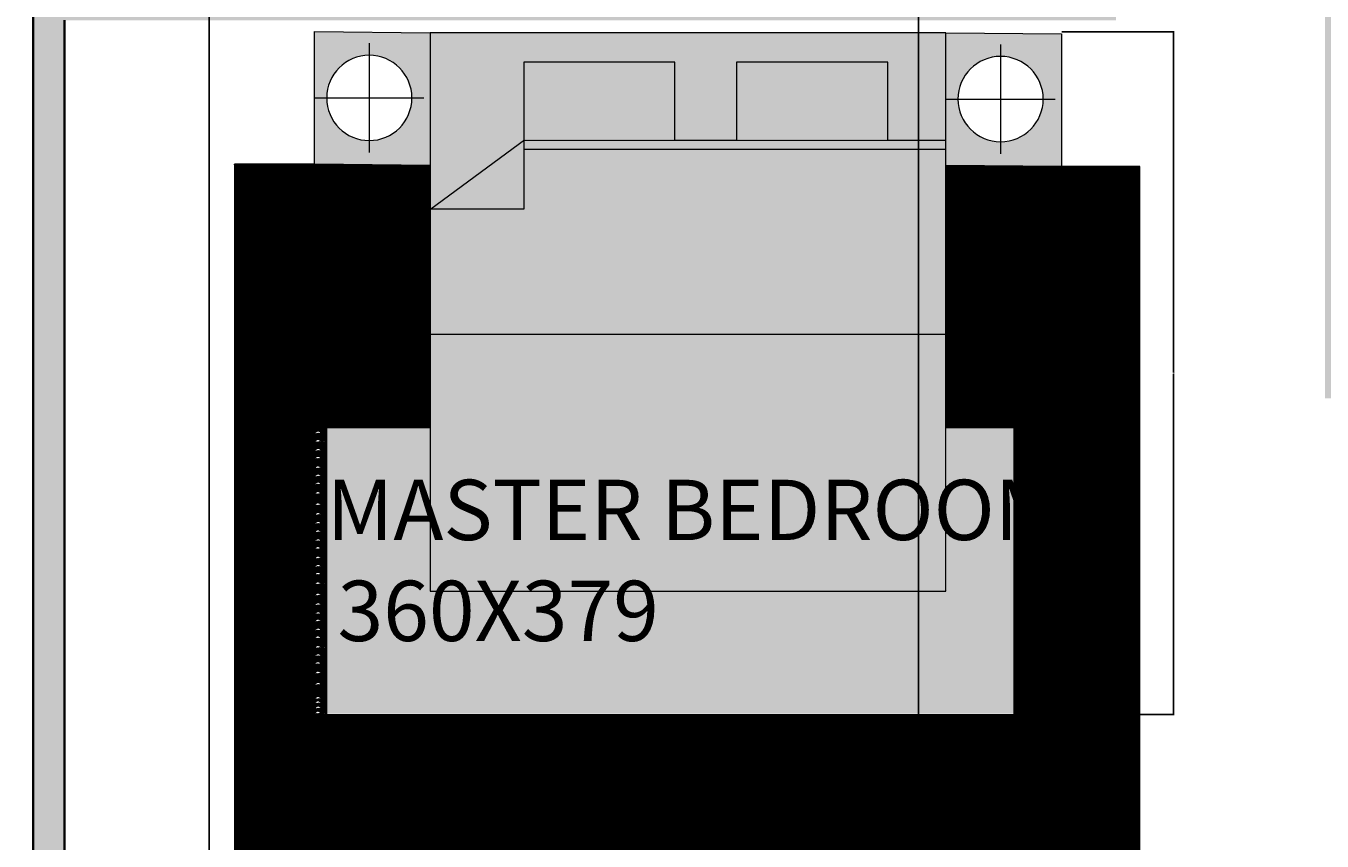
# Model space of a CAD drawing. Units: inches. Extents: x 192 to 1361, y -1362 to 367.
# Tile 21 of 23: x 783 to 1153, y -304 to -71. Entities that reach past the tile are written whole.
import ezdxf

# ---------------------------------------------------------------- set-up
doc = ezdxf.new("R2010")
doc.units = ezdxf.units.IN
doc.header["$MEASUREMENT"] = 0
for name, color, linetype, lineweight in [('A-ANNO-DIMS', 2, 'Continuous', 18), ('A-AREA-IDEN', 7, 'Continuous', 18), ('A-FLOR', 8, 'Continuous', 18), ('A-WALL-PATT', 250, 'Continuous', 13), ('furniture', 32, 'Continuous', 18), ('walls', 7, 'Continuous', 35)]:
    doc.layers.add(name, color=color, linetype=linetype, lineweight=lineweight)
doc.layers.add('A-FLOR-PATT', color=254, linetype='Continuous', lineweight=13, true_color=0xfeeab9)
doc.layers.add('A-FURN-PATT', color=254, linetype='Continuous', lineweight=13, true_color=0xfeeab9)
doc.styles.get("Standard").update_dxf_attribs({"font": 'arial.ttf'})
doc.dimstyles.get("Standard").update_dxf_attribs({"dimtxt": 0.18, "dimasz": 0.18, "dimexe": 0.18, "dimexo": 0.0625, "dimgap": 0.09, "dimtad": 0, "dimtih": 1, "dimtoh": 1, "dimzin": 0, "dimdsep": 46, "dimlunit": 3, "dimtxsty": 'Standard', "dimcen": 0.09, "dimadec": 0, "dimazin": 0, "dimtfac": 1, "dimtofl": 0, "dimtmove": 0, "dimatfit": 3, "dimfxl": 1, "dimtolj": 1, "dimtzin": 0, "dimarcsym": 0})

# ---------------------------------------------------------------- blocks, each defined once
blk = doc.blocks.new('CARPET')
at = {"layer": 'furniture'}
for p, q in [((-51.53, -98.11), (-51.53, -55.12)), ((-51.53, -55.12), (-41.27, -55.12)), ((36, -55.12), (51.55, -55.12)), ((51.55, -55.12), (51.55, -98.11)), ((51.55, -98.11), (-51.53, -98.11))]:
    blk.add_line(p, q, dxfattribs=at)
for points, knots in [([(-53.37, -55.99), (-53.22, -55.8), (-52.9, -55.41), (-52.34, -55.8), (-51.89, -56.08), (-51.65, -55.91), (-51.53, -55.83)], [0, 0, 0, 0, 0.653278, 1.290138, 1.740457, 2.114451, 2.114451, 2.114451, 2.114451]), ([(53.37, -55.99), (53.22, -55.8), (52.9, -55.41), (52.34, -55.8), (51.89, -56.08), (51.65, -55.91), (51.53, -55.83)], [0, 0, 0, 0, 0.653278, 1.290138, 1.740457, 2.114451, 2.114451, 2.114451, 2.114451]), ([(-53.37, -57.26), (-53.22, -57.07), (-52.9, -56.67), (-52.34, -57.07), (-51.89, -57.35), (-51.65, -57.17), (-51.53, -57.1)], [0, 0, 0, 0, 0.653278, 1.290138, 1.740457, 2.114451, 2.114451, 2.114451, 2.114451]), ([(-53.37, -58.59), (-53.22, -58.4), (-52.9, -58.01), (-52.34, -58.4), (-51.89, -58.68), (-51.65, -58.5), (-51.53, -58.43)], [0, 0, 0, 0, 0.653278, 1.290138, 1.740457, 2.114451, 2.114451, 2.114451, 2.114451]), ([(53.37, -57.26), (53.22, -57.07), (52.9, -56.67), (52.34, -57.07), (51.89, -57.35), (51.65, -57.17), (51.53, -57.1)], [0, 0, 0, 0, 0.653278, 1.290138, 1.740457, 2.114451, 2.114451, 2.114451, 2.114451]), ([(53.37, -58.59), (53.22, -58.4), (52.9, -58.01), (52.34, -58.4), (51.89, -58.68), (51.65, -58.5), (51.53, -58.43)], [0, 0, 0, 0, 0.653278, 1.290138, 1.740457, 2.114451, 2.114451, 2.114451, 2.114451]), ([(-53.37, -59.78), (-53.22, -59.58), (-52.9, -59.19), (-52.34, -59.58), (-51.89, -59.86), (-51.65, -59.69), (-51.53, -59.61)], [0, 0, 0, 0, 0.653278, 1.290138, 1.740457, 2.114451, 2.114451, 2.114451, 2.114451]), ([(53.37, -59.78), (53.22, -59.58), (52.9, -59.19), (52.34, -59.58), (51.89, -59.86), (51.65, -59.69), (51.53, -59.61)], [0, 0, 0, 0, 0.653278, 1.290138, 1.740457, 2.114451, 2.114451, 2.114451, 2.114451]), ([(-53.37, -61.22), (-53.22, -61.02), (-52.9, -60.63), (-52.34, -61.02), (-51.89, -61.3), (-51.65, -61.13), (-51.53, -61.05)], [0, 0, 0, 0, 0.653278, 1.290138, 1.740457, 2.114451, 2.114451, 2.114451, 2.114451]), ([(-53.37, -62.44), (-53.22, -62.25), (-52.9, -61.86), (-52.34, -62.25), (-51.89, -62.53), (-51.65, -62.36), (-51.53, -62.28)], [0, 0, 0, 0, 0.653278, 1.290138, 1.740457, 2.114451, 2.114451, 2.114451, 2.114451]), ([(53.37, -61.22), (53.22, -61.02), (52.9, -60.63), (52.34, -61.02), (51.89, -61.3), (51.65, -61.13), (51.53, -61.05)], [0, 0, 0, 0, 0.653278, 1.290138, 1.740457, 2.114451, 2.114451, 2.114451, 2.114451]), ([(53.37, -62.44), (53.22, -62.25), (52.9, -61.86), (52.34, -62.25), (51.89, -62.53), (51.65, -62.36), (51.53, -62.28)], [0, 0, 0, 0, 0.653278, 1.290138, 1.740457, 2.114451, 2.114451, 2.114451, 2.114451]), ([(-53.37, -63.63), (-53.22, -63.43), (-52.9, -63.04), (-52.34, -63.43), (-51.89, -63.72), (-51.65, -63.54), (-51.53, -63.46)], [0, 0, 0, 0, 0.653278, 1.290138, 1.740457, 2.114451, 2.114451, 2.114451, 2.114451]), ([(53.37, -63.63), (53.22, -63.43), (52.9, -63.04), (52.34, -63.43), (51.89, -63.72), (51.65, -63.54), (51.53, -63.46)], [0, 0, 0, 0, 0.653278, 1.290138, 1.740457, 2.114451, 2.114451, 2.114451, 2.114451]), ([(-53.37, -65.07), (-53.22, -64.87), (-52.9, -64.48), (-52.34, -64.87), (-51.89, -65.15), (-51.65, -64.98), (-51.53, -64.9)], [0, 0, 0, 0, 0.653278, 1.290138, 1.740457, 2.114451, 2.114451, 2.114451, 2.114451]), ([(53.37, -65.07), (53.22, -64.87), (52.9, -64.48), (52.34, -64.87), (51.89, -65.15), (51.65, -64.98), (51.53, -64.9)], [0, 0, 0, 0, 0.653278, 1.290138, 1.740457, 2.114451, 2.114451, 2.114451, 2.114451]), ([(-53.37, -66.76), (-53.22, -66.56), (-52.9, -66.17), (-52.34, -66.56), (-51.89, -66.84), (-51.65, -66.67), (-51.53, -66.59)], [0, 0, 0, 0, 0.653278, 1.290138, 1.740457, 2.114451, 2.114451, 2.114451, 2.114451]), ([(-53.37, -68.2), (-53.22, -68), (-52.9, -67.61), (-52.34, -68), (-51.89, -68.28), (-51.65, -68.11), (-51.53, -68.03)], [0, 0, 0, 0, 0.653278, 1.290138, 1.740457, 2.114451, 2.114451, 2.114451, 2.114451]), ([(53.37, -66.76), (53.22, -66.56), (52.9, -66.17), (52.34, -66.56), (51.89, -66.84), (51.65, -66.67), (51.53, -66.59)], [0, 0, 0, 0, 0.653278, 1.290138, 1.740457, 2.114451, 2.114451, 2.114451, 2.114451]), ([(53.37, -68.2), (53.22, -68), (52.9, -67.61), (52.34, -68), (51.89, -68.28), (51.65, -68.11), (51.53, -68.03)], [0, 0, 0, 0, 0.653278, 1.290138, 1.740457, 2.114451, 2.114451, 2.114451, 2.114451]), ([(-53.37, -69.53), (-53.22, -69.33), (-52.9, -68.94), (-52.34, -69.33), (-51.89, -69.61), (-51.65, -69.44), (-51.53, -69.36)], [0, 0, 0, 0, 0.653278, 1.290138, 1.740457, 2.114451, 2.114451, 2.114451, 2.114451]), ([(53.37, -69.53), (53.22, -69.33), (52.9, -68.94), (52.34, -69.33), (51.89, -69.61), (51.65, -69.44), (51.53, -69.36)], [0, 0, 0, 0, 0.653278, 1.290138, 1.740457, 2.114451, 2.114451, 2.114451, 2.114451]), ([(-53.37, -70.79), (-53.22, -70.6), (-52.9, -70.21), (-52.34, -70.6), (-51.89, -70.88), (-51.65, -70.7), (-51.53, -70.63)], [0, 0, 0, 0, 0.653278, 1.290138, 1.740457, 2.114451, 2.114451, 2.114451, 2.114451]), ([(-53.37, -72.12), (-53.22, -71.93), (-52.9, -71.54), (-52.34, -71.93), (-51.89, -72.21), (-51.65, -72.04), (-51.53, -71.96)], [0, 0, 0, 0, 0.653278, 1.290138, 1.740457, 2.114451, 2.114451, 2.114451, 2.114451]), ([(53.37, -70.79), (53.22, -70.6), (52.9, -70.21), (52.34, -70.6), (51.89, -70.88), (51.65, -70.7), (51.53, -70.63)], [0, 0, 0, 0, 0.653278, 1.290138, 1.740457, 2.114451, 2.114451, 2.114451, 2.114451]), ([(53.37, -72.12), (53.22, -71.93), (52.9, -71.54), (52.34, -71.93), (51.89, -72.21), (51.65, -72.04), (51.53, -71.96)], [0, 0, 0, 0, 0.653278, 1.290138, 1.740457, 2.114451, 2.114451, 2.114451, 2.114451]), ([(-53.37, -73.31), (-53.22, -73.11), (-52.9, -72.72), (-52.34, -73.11), (-51.89, -73.4), (-51.65, -73.22), (-51.53, -73.14)], [0, 0, 0, 0, 0.653278, 1.290138, 1.740457, 2.114451, 2.114451, 2.114451, 2.114451]), ([(53.37, -73.31), (53.22, -73.11), (52.9, -72.72), (52.34, -73.11), (51.89, -73.4), (51.65, -73.22), (51.53, -73.14)], [0, 0, 0, 0, 0.653278, 1.290138, 1.740457, 2.114451, 2.114451, 2.114451, 2.114451]), ([(-53.37, -74.75), (-53.22, -74.55), (-52.9, -74.16), (-52.34, -74.55), (-51.89, -74.83), (-51.65, -74.66), (-51.53, -74.58)], [0, 0, 0, 0, 0.653278, 1.290138, 1.740457, 2.114451, 2.114451, 2.114451, 2.114451]), ([(-53.37, -75.98), (-53.22, -75.78), (-52.9, -75.39), (-52.34, -75.78), (-51.89, -76.06), (-51.65, -75.89), (-51.53, -75.81)], [0, 0, 0, 0, 0.653278, 1.290138, 1.740457, 2.114451, 2.114451, 2.114451, 2.114451]), ([(53.37, -74.75), (53.22, -74.55), (52.9, -74.16), (52.34, -74.55), (51.89, -74.83), (51.65, -74.66), (51.53, -74.58)], [0, 0, 0, 0, 0.653278, 1.290138, 1.740457, 2.114451, 2.114451, 2.114451, 2.114451]), ([(53.37, -75.98), (53.22, -75.78), (52.9, -75.39), (52.34, -75.78), (51.89, -76.06), (51.65, -75.89), (51.53, -75.81)], [0, 0, 0, 0, 0.653278, 1.290138, 1.740457, 2.114451, 2.114451, 2.114451, 2.114451]), ([(-53.37, -77.16), (-53.22, -76.96), (-52.9, -76.57), (-52.34, -76.96), (-51.89, -77.25), (-51.65, -77.07), (-51.53, -76.99)], [0, 0, 0, 0, 0.653278, 1.290138, 1.740457, 2.114451, 2.114451, 2.114451, 2.114451]), ([(53.37, -77.16), (53.22, -76.96), (52.9, -76.57), (52.34, -76.96), (51.89, -77.25), (51.65, -77.07), (51.53, -76.99)], [0, 0, 0, 0, 0.653278, 1.290138, 1.740457, 2.114451, 2.114451, 2.114451, 2.114451]), ([(-53.37, -78.6), (-53.22, -78.4), (-52.9, -78.01), (-52.34, -78.4), (-51.89, -78.68), (-51.65, -78.51), (-51.53, -78.43)], [0, 0, 0, 0, 0.653278, 1.290138, 1.740457, 2.114451, 2.114451, 2.114451, 2.114451]), ([(53.37, -78.6), (53.22, -78.4), (52.9, -78.01), (52.34, -78.4), (51.89, -78.68), (51.65, -78.51), (51.53, -78.43)], [0, 0, 0, 0, 0.653278, 1.290138, 1.740457, 2.114451, 2.114451, 2.114451, 2.114451]), ([(-53.37, -80.29), (-53.22, -80.09), (-52.9, -79.7), (-52.34, -80.09), (-51.89, -80.37), (-51.65, -80.2), (-51.53, -80.12)], [0, 0, 0, 0, 0.653278, 1.290138, 1.740457, 2.114451, 2.114451, 2.114451, 2.114451]), ([(-53.37, -81.73), (-53.22, -81.53), (-52.9, -81.14), (-52.34, -81.53), (-51.89, -81.81), (-51.65, -81.64), (-51.53, -81.56)], [0, 0, 0, 0, 0.653278, 1.290138, 1.740457, 2.114451, 2.114451, 2.114451, 2.114451]), ([(53.37, -80.29), (53.22, -80.09), (52.9, -79.7), (52.34, -80.09), (51.89, -80.37), (51.65, -80.2), (51.53, -80.12)], [0, 0, 0, 0, 0.653278, 1.290138, 1.740457, 2.114451, 2.114451, 2.114451, 2.114451]), ([(53.37, -81.73), (53.22, -81.53), (52.9, -81.14), (52.34, -81.53), (51.89, -81.81), (51.65, -81.64), (51.53, -81.56)], [0, 0, 0, 0, 0.653278, 1.290138, 1.740457, 2.114451, 2.114451, 2.114451, 2.114451]), ([(-53.37, -83.06), (-53.22, -82.86), (-52.9, -82.47), (-52.34, -82.86), (-51.89, -83.14), (-51.65, -82.97), (-51.53, -82.89)], [0, 0, 0, 0, 0.653278, 1.290138, 1.740457, 2.114451, 2.114451, 2.114451, 2.114451]), ([(53.37, -83.06), (53.22, -82.86), (52.9, -82.47), (52.34, -82.86), (51.89, -83.14), (51.65, -82.97), (51.53, -82.89)], [0, 0, 0, 0, 0.653278, 1.290138, 1.740457, 2.114451, 2.114451, 2.114451, 2.114451]), ([(-53.37, -84.18), (-53.22, -83.99), (-52.9, -83.6), (-52.34, -83.99), (-51.89, -84.27), (-51.65, -84.09), (-51.53, -84.02)], [0, 0, 0, 0, 0.653278, 1.290138, 1.740457, 2.114451, 2.114451, 2.114451, 2.114451]), ([(-53.37, -85.51), (-53.22, -85.32), (-52.9, -84.93), (-52.34, -85.32), (-51.89, -85.6), (-51.65, -85.42), (-51.53, -85.35)], [0, 0, 0, 0, 0.653278, 1.290138, 1.740457, 2.114451, 2.114451, 2.114451, 2.114451]), ([(53.37, -84.18), (53.22, -83.99), (52.9, -83.6), (52.34, -83.99), (51.89, -84.27), (51.65, -84.09), (51.53, -84.02)], [0, 0, 0, 0, 0.653278, 1.290138, 1.740457, 2.114451, 2.114451, 2.114451, 2.114451]), ([(53.37, -85.51), (53.22, -85.32), (52.9, -84.93), (52.34, -85.32), (51.89, -85.6), (51.65, -85.42), (51.53, -85.35)], [0, 0, 0, 0, 0.653278, 1.290138, 1.740457, 2.114451, 2.114451, 2.114451, 2.114451]), ([(-53.37, -86.7), (-53.22, -86.5), (-52.9, -86.11), (-52.34, -86.5), (-51.89, -86.78), (-51.65, -86.61), (-51.53, -86.53)], [0, 0, 0, 0, 0.653278, 1.290138, 1.740457, 2.114451, 2.114451, 2.114451, 2.114451]), ([(53.37, -86.7), (53.22, -86.5), (52.9, -86.11), (52.34, -86.5), (51.89, -86.78), (51.65, -86.61), (51.53, -86.53)], [0, 0, 0, 0, 0.653278, 1.290138, 1.740457, 2.114451, 2.114451, 2.114451, 2.114451]), ([(-53.37, -88.14), (-53.22, -87.94), (-52.9, -87.55), (-52.34, -87.94), (-51.89, -88.22), (-51.65, -88.05), (-51.53, -87.97)], [0, 0, 0, 0, 0.653278, 1.290138, 1.740457, 2.114451, 2.114451, 2.114451, 2.114451]), ([(-53.37, -89.36), (-53.22, -89.17), (-52.9, -88.78), (-52.34, -89.17), (-51.89, -89.45), (-51.65, -89.28), (-51.53, -89.2)], [0, 0, 0, 0, 0.653278, 1.290138, 1.740457, 2.114451, 2.114451, 2.114451, 2.114451]), ([(53.37, -88.14), (53.22, -87.94), (52.9, -87.55), (52.34, -87.94), (51.89, -88.22), (51.65, -88.05), (51.53, -87.97)], [0, 0, 0, 0, 0.653278, 1.290138, 1.740457, 2.114451, 2.114451, 2.114451, 2.114451]), ([(53.37, -89.36), (53.22, -89.17), (52.9, -88.78), (52.34, -89.17), (51.89, -89.45), (51.65, -89.28), (51.53, -89.2)], [0, 0, 0, 0, 0.653278, 1.290138, 1.740457, 2.114451, 2.114451, 2.114451, 2.114451]), ([(-53.37, -90.55), (-53.22, -90.35), (-52.9, -89.96), (-52.34, -90.35), (-51.89, -90.64), (-51.65, -90.46), (-51.53, -90.38)], [0, 0, 0, 0, 0.653278, 1.290138, 1.740457, 2.114451, 2.114451, 2.114451, 2.114451]), ([(53.37, -90.55), (53.22, -90.35), (52.9, -89.96), (52.34, -90.35), (51.9, -90.63), (51.66, -90.47), (51.55, -90.4)], [0, 0, 0, 0, 0.653278, 1.290138, 1.740457, 2.0926, 2.0926, 2.0926, 2.0926]), ([(-53.37, -91.99), (-53.22, -91.79), (-52.9, -91.4), (-52.34, -91.79), (-51.89, -92.07), (-51.65, -91.9), (-51.53, -91.82)], [0, 0, 0, 0, 0.653278, 1.290138, 1.740457, 2.114451, 2.114451, 2.114451, 2.114451]), ([(-53.37, -92.69), (-53.22, -92.48), (-52.9, -92.08), (-52.35, -92.49), (-51.89, -92.77), (-51.65, -92.6), (-51.53, -92.52)], [0, 0, 0, 0, 0.663904, 1.307406, 1.757725, 2.131719, 2.131719, 2.131719, 2.131719]), ([(-53.37, -93.61), (-53.22, -93.42), (-52.9, -93.03), (-52.34, -93.42), (-51.89, -93.7), (-51.65, -93.52), (-51.53, -93.45)], [0, 0, 0, 0, 0.653278, 1.290138, 1.740457, 2.114451, 2.114451, 2.114451, 2.114451]), ([(53.37, -91.99), (53.22, -91.79), (52.9, -91.4), (52.34, -91.79), (51.9, -92.07), (51.66, -91.91), (51.55, -91.83)], [0, 0, 0, 0, 0.653278, 1.290138, 1.740457, 2.0926, 2.0926, 2.0926, 2.0926]), ([(53.37, -92.69), (53.22, -92.49), (52.9, -92.09), (52.34, -92.49), (51.9, -92.77), (51.66, -92.61), (51.55, -92.53)], [0, 0, 0, 0, 0.656792, 1.295826, 1.746145, 2.098292, 2.098292, 2.098292, 2.098292]), ([(53.37, -93.66), (53.22, -93.46), (52.9, -93.07), (52.34, -93.46), (51.9, -93.74), (51.66, -93.58), (51.55, -93.5)], [0, 0, 0, 0, 0.653278, 1.290138, 1.740457, 2.0926, 2.0926, 2.0926, 2.0926]), ([(-53.37, -94.55), (-53.22, -94.35), (-52.9, -93.96), (-52.34, -94.35), (-51.89, -94.63), (-51.65, -94.46), (-51.53, -94.38)], [0, 0, 0, 0, 0.653278, 1.290138, 1.740457, 2.114451, 2.114451, 2.114451, 2.114451]), ([(-53.37, -95.05), (-53.22, -94.85), (-52.9, -94.46), (-52.34, -94.85), (-51.89, -95.14), (-51.65, -94.96), (-51.53, -94.88)], [0, 0, 0, 0, 0.653278, 1.290138, 1.740457, 2.114451, 2.114451, 2.114451, 2.114451]), ([(53.37, -94.59), (53.22, -94.4), (52.9, -94.01), (52.34, -94.4), (51.9, -94.68), (51.66, -94.51), (51.55, -94.44)], [0, 0, 0, 0, 0.653278, 1.290138, 1.740457, 2.0926, 2.0926, 2.0926, 2.0926]), ([(53.37, -95.1), (53.22, -94.9), (52.9, -94.51), (52.34, -94.9), (51.9, -95.18), (51.66, -95.02), (51.55, -94.94)], [0, 0, 0, 0, 0.653278, 1.290138, 1.740457, 2.0926, 2.0926, 2.0926, 2.0926]), ([(-53.37, -95.73), (-53.22, -95.54), (-52.9, -95.15), (-52.34, -95.54), (-51.89, -95.82), (-51.65, -95.65), (-51.53, -95.57)], [0, 0, 0, 0, 0.653278, 1.290138, 1.740457, 2.114451, 2.114451, 2.114451, 2.114451]), ([(-53.37, -96.38), (-53.22, -96.18), (-52.9, -95.79), (-52.34, -96.18), (-51.89, -96.47), (-51.65, -96.29), (-51.53, -96.21)], [0, 0, 0, 0, 0.653278, 1.290138, 1.740457, 2.114451, 2.114451, 2.114451, 2.114451]), ([(-53.37, -97.17), (-53.22, -96.98), (-52.9, -96.59), (-52.34, -96.98), (-51.89, -97.26), (-51.65, -97.08), (-51.53, -97.01)], [0, 0, 0, 0, 0.653278, 1.290138, 1.740457, 2.114451, 2.114451, 2.114451, 2.114451]), ([(53.37, -95.78), (53.22, -95.58), (52.9, -95.19), (52.34, -95.58), (51.89, -95.86), (51.65, -95.69), (51.53, -95.61)], [0, 0, 0, 0, 0.653278, 1.290138, 1.740457, 2.114451, 2.114451, 2.114451, 2.114451]), ([(53.37, -96.43), (53.22, -96.23), (52.9, -95.84), (52.34, -96.23), (51.89, -96.51), (51.65, -96.34), (51.53, -96.26)], [0, 0, 0, 0, 0.653278, 1.290138, 1.740457, 2.114451, 2.114451, 2.114451, 2.114451]), ([(53.37, -97.22), (53.22, -97.02), (52.9, -96.63), (52.34, -97.02), (51.89, -97.3), (51.65, -97.13), (51.53, -97.05)], [0, 0, 0, 0, 0.653278, 1.290138, 1.740457, 2.114451, 2.114451, 2.114451, 2.114451]), ([(-53.37, -97.99), (-53.22, -97.79), (-52.9, -97.4), (-52.34, -97.79), (-51.89, -98.08), (-51.65, -97.9), (-51.53, -97.82)], [0, 0, 0, 0, 0.653278, 1.290138, 1.740457, 2.114451, 2.114451, 2.114451, 2.114451]), ([(53.37, -97.99), (53.22, -97.79), (52.9, -97.4), (52.34, -97.79), (51.89, -98.08), (51.65, -97.9), (51.53, -97.82)], [0, 0, 0, 0, 0.653278, 1.290138, 1.740457, 2.114451, 2.114451, 2.114451, 2.114451])]:
    blk.add_open_spline(points, degree=3, knots=knots, dxfattribs=at)
blk = doc.blocks.new('A$C58D270C6')
at = {"layer": 'furniture'}
for p, q in [((9.09, 124.13), (9.09, 108.87)), ((1.46, 116.5), (16.73, 116.5)), ((14.97, 94.84), (24.62, 107.92)), ((24.62, 94.93), (24.62, 107.92)), ((42.08, 108), (42.08, 36)), ((14.97, 94.93), (24.62, 94.93)), ((14.97, 94.84), (14.97, 36)), ((16.22, 94.93), (16.22, 36)), ((9.25, 36), (9.25, 20.74)), ((1.62, 28.37), (16.88, 28.37))]:
    blk.add_line(p, q, dxfattribs=at)
for points in [[(18.5, 108), (18.34, 124.13), (-0.16, 124.13), (0, 108)], [(0, 108), (77.91, 108), (77.91, 36), (0, 36)], [(4.09, 94.93), (14.97, 94.93), (14.97, 73.83), (4.09, 73.83)], [(4.09, 65.23), (14.97, 65.23), (14.97, 44.13), (4.09, 44.13)], [(18.65, 19.87), (18.5, 36), (0, 36), (0.16, 19.87)]]:
    blk.add_lwpolyline(points, close=True, dxfattribs=at)
for centre in [(9.09, 116.5), (9.25, 28.37)]:
    blk.add_circle(centre, 5.95, dxfattribs=at)
at = {"layer": 'furniture', "xscale": 0.9312884925094044, "yscale": 0.9312884925094044, "zscale": 0.9312884925094044, "rotation": 90}
blk.add_blockref('CARPET', (3.79, 74.47), dxfattribs=at)
blk = doc.blocks.new('*D25')
at = {"layer": 'A-ANNO-DIMS', "color": 0, "lineweight": -2, "transparency": 16777216}
for p, q in [((865.12, -267.87), (865.12, -300)), ((1078.56, -267.87), (1078.56, -300)), ((865.3, -299.82), (971.26, -299.82)), ((1078.38, -299.82), (972.42, -299.82))]:
    blk.add_line(p, q, dxfattribs=at)
at = {"layer": 'A-ANNO-DIMS', "color": 0, "transparency": 16777216}
for points in [[(865.3, -299.79), (865.3, -299.85), (865.12, -299.82)], [(1078.38, -299.79), (1078.38, -299.85), (1078.56, -299.82)]]:
    blk.add_solid(points, dxfattribs=at)
at = {"layer": 'Defpoints', "color": 0, "transparency": 16777216}
for p in [(865.12, -267.81), (1078.56, -267.81), (865.12, -299.82)]:
    blk.add_point(p, dxfattribs=at)
at = {"layer": 'A-ANNO-DIMS', "color": 0, "transparency": 16777216, "insert": (971.84, -299.82), "char_height": 0.18, "attachment_point": 5}
blk.add_mtext('\\A1;BED 213', dxfattribs=at)
blk = doc.blocks.new('*D26')
at = {"layer": 'A-ANNO-DIMS', "color": 0, "lineweight": -2, "transparency": 16777216}
for p, q in [((1078.62, -72.78), (1110.76, -72.78)), ((1110.58, -72.96), (1110.58, -170.11)), ((1110.58, -267.63), (1110.58, -170.47)), ((1078.62, -267.81), (1110.76, -267.81))]:
    blk.add_line(p, q, dxfattribs=at)
at = {"layer": 'A-ANNO-DIMS', "color": 0, "transparency": 16777216}
for points in [[(1110.55, -72.96), (1110.61, -72.96), (1110.58, -72.78)], [(1110.55, -267.63), (1110.61, -267.63), (1110.58, -267.81)]]:
    blk.add_solid(points, dxfattribs=at)
at = {"layer": 'Defpoints', "color": 0, "transparency": 16777216}
for p in [(1078.56, -72.78), (1078.56, -267.81), (1110.58, -267.81)]:
    blk.add_point(p, dxfattribs=at)
at = {"layer": 'A-ANNO-DIMS', "color": 0, "transparency": 16777216, "insert": (1110.58, -170.29), "char_height": 0.18, "attachment_point": 5}
blk.add_mtext('\\A1;195', dxfattribs=at)
blk = doc.blocks.new('*D72')
at = {"layer": 'A-ANNO-DIMS', "color": 0, "lineweight": -2, "transparency": 16777216}
for p, q in [((835.08, -1067.56), (835.08, 367.39)), ((835.26, 367.21), (935.95, 367.21)), ((1037.58, 367.21), (936.88, 367.21)), ((1037.76, -1067.56), (1037.76, 367.39))]:
    blk.add_line(p, q, dxfattribs=at)
at = {"layer": 'A-ANNO-DIMS', "color": 0, "transparency": 16777216}
for points in [[(835.26, 367.24), (835.26, 367.18), (835.08, 367.21)], [(1037.58, 367.24), (1037.58, 367.18), (1037.76, 367.21)]]:
    blk.add_solid(points, dxfattribs=at)
at = {"layer": 'Defpoints', "color": 0, "transparency": 16777216}
for p in [(1037.76, 367.21), (835.08, -1067.62), (1037.76, -1067.62)]:
    blk.add_point(p, dxfattribs=at)
at = {"layer": 'A-ANNO-DIMS', "color": 0, "transparency": 16777216, "insert": (936.42, 367.21), "char_height": 0.18, "attachment_point": 5}
blk.add_mtext('\\A1;202.68', dxfattribs=at)

msp = doc.modelspace()

# ---------------------------------------------------------------- hatches: boundary and pattern name
at = {"layer": 'A-FLOR-PATT'}
h = msp.add_hatch(dxfattribs=at)
h.set_pattern_fill('ANSI31', color=256)
edge = h.paths.add_edge_path()
edge.add_line((1100.9659, -111.2666), (1078.5607, -111.2666))
edge.add_line((1078.5607, -111.2666), (1045.5537, -110.9483))
edge.add_line((1045.5537, -110.9483), (1045.5537, -185.8956))
edge.add_line((1045.5537, -185.8956), (1065.0331, -185.8956))
edge.add_line((1065.0331, -185.8956), (1065.0331, -267.8066))
edge.add_line((1065.0331, -267.8066), (868.5929, -267.8066))
edge.add_line((868.5929, -267.8066), (868.5929, -267.2863))
edge.add_spline(control_points=[(865.1222, -267.5809), (865.4243, -267.2044), (866.0209, -266.461), (867.0867, -267.2043), (867.9397, -267.7344), (868.3935, -267.4276), (868.5929, -267.2863)], knot_values=[0, 0, 0, 0, 0.65327829, 1.2901376, 1.74045698, 2.09412198, 2.09412198, 2.09412198, 2.09412198], degree=3, periodic=0)
edge.add_line((868.5929, -267.2863), (868.5929, -265.8146))
edge.add_spline(control_points=[(865.1222, -266.1092), (865.4243, -265.7327), (866.0209, -264.9893), (867.0867, -265.7326), (867.9397, -266.2626), (868.3935, -265.9559), (868.5929, -265.8146)], knot_values=[0, 0, 0, 0, 0.65327829, 1.2901376, 1.74045698, 2.09412198, 2.09412198, 2.09412198, 2.09412198], degree=3, periodic=0)
edge.add_line((868.5929, -265.8146), (868.5929, -264.3081))
edge.add_spline(control_points=[(865.1222, -264.6026), (865.4243, -264.2262), (866.0209, -263.4827), (867.0867, -264.2261), (867.9397, -264.7561), (868.3935, -264.4493), (868.5929, -264.3081)], knot_values=[0, 0, 0, 0, 0.65327829, 1.2901376, 1.74045698, 2.09412198, 2.09412198, 2.09412198, 2.09412198], degree=3, periodic=0)
edge.add_line((868.5929, -264.3081), (868.5929, -263.0738))
edge.add_spline(control_points=[(865.1222, -263.3684), (865.4243, -262.9919), (866.0209, -262.2485), (867.0867, -262.9918), (867.9397, -263.5219), (868.3935, -263.2151), (868.5929, -263.0738)], knot_values=[0, 0, 0, 0, 0.65327829, 1.2901376, 1.74045698, 2.09412198, 2.09412198, 2.09412198, 2.09412198], degree=3, periodic=0)
edge.add_line((868.5929, -263.0738), (868.5929, -259.0322))
edge.add_spline(control_points=[(865.1222, -259.3268), (865.4242, -258.9505), (866.0208, -258.2073), (867.0871, -258.949), (867.938, -259.4827), (868.3932, -259.1696), (868.5929, -259.0322)], knot_values=[0, 0, 0, 0, 0.65327829, 1.2901376, 1.74045698, 2.09260048, 2.09260048, 2.09260048, 2.09260048], degree=3, periodic=0)
edge.add_line((868.5929, -259.0322), (868.5929, -255.8497))
edge.add_spline(control_points=[(865.1222, -256.1443), (865.4242, -255.768), (866.0208, -255.0247), (867.0871, -255.7664), (867.938, -256.3002), (868.3932, -255.9871), (868.5929, -255.8497)], knot_values=[0, 0, 0, 0, 0.65327829, 1.2901376, 1.74045698, 2.09260048, 2.09260048, 2.09260048, 2.09260048], degree=3, periodic=0)
edge.add_line((868.5929, -255.8497), (868.5929, -253.1089))
edge.add_spline(control_points=[(865.1222, -253.4035), (865.4242, -253.0272), (866.0208, -252.284), (867.0871, -253.0257), (867.938, -253.5594), (868.3932, -253.2463), (868.5929, -253.1089)], knot_values=[0, 0, 0, 0, 0.65327829, 1.2901376, 1.74045698, 2.09260048, 2.09260048, 2.09260048, 2.09260048], degree=3, periodic=0)
edge.add_line((868.5929, -253.1089), (868.5929, -250.8478))
edge.add_spline(control_points=[(865.1222, -251.1424), (865.4243, -250.766), (866.0209, -250.0225), (867.0867, -250.7659), (867.9397, -251.2959), (868.3935, -250.9891), (868.5929, -250.8478)], knot_values=[0, 0, 0, 0, 0.65327829, 1.2901376, 1.74045698, 2.09412198, 2.09412198, 2.09412198, 2.09412198], degree=3, periodic=0)
edge.add_line((868.5929, -250.8478), (868.5929, -248.511))
edge.add_spline(control_points=[(865.1222, -248.8056), (865.4243, -248.4291), (866.0209, -247.6857), (867.0867, -248.429), (867.9397, -248.9591), (868.3935, -248.6523), (868.5929, -248.511)], knot_values=[0, 0, 0, 0, 0.65327829, 1.2901376, 1.74045698, 2.09412198, 2.09412198, 2.09412198, 2.09412198], degree=3, periodic=0)
edge.add_line((868.5929, -248.511), (868.5929, -245.7702))
edge.add_spline(control_points=[(865.1222, -246.0648), (865.4243, -245.6884), (866.0209, -244.9449), (867.0867, -245.6883), (867.9397, -246.2183), (868.3935, -245.9115), (868.5929, -245.7702)], knot_values=[0, 0, 0, 0, 0.65327829, 1.2901376, 1.74045698, 2.09412198, 2.09412198, 2.09412198, 2.09412198], degree=3, periodic=0)
edge.add_line((868.5929, -245.7702), (868.5929, -243.5091))
edge.add_spline(control_points=[(865.1222, -243.8037), (865.4243, -243.4273), (866.0209, -242.6838), (867.0867, -243.4272), (867.9397, -243.9572), (868.3935, -243.6504), (868.5929, -243.5091)], knot_values=[0, 0, 0, 0, 0.65327829, 1.2901376, 1.74045698, 2.09412198, 2.09412198, 2.09412198, 2.09412198], degree=3, periodic=0)
edge.add_line((868.5929, -243.5091), (868.5929, -240.974))
edge.add_spline(control_points=[(865.1222, -241.2686), (865.4243, -240.8921), (866.0209, -240.1487), (867.0867, -240.892), (867.9397, -241.422), (868.3935, -241.1153), (868.5929, -240.974)], knot_values=[0, 0, 0, 0, 0.65327829, 1.2901376, 1.74045698, 2.09412198, 2.09412198, 2.09412198, 2.09412198], degree=3, periodic=0)
edge.add_line((868.5929, -240.974), (868.5929, -238.832))
edge.add_spline(control_points=[(865.1222, -239.1266), (865.4243, -238.7501), (866.0209, -238.0067), (867.0867, -238.75), (867.9397, -239.2801), (868.3935, -238.9733), (868.5929, -238.832)], knot_values=[0, 0, 0, 0, 0.65327829, 1.2901376, 1.74045698, 2.09412198, 2.09412198, 2.09412198, 2.09412198], degree=3, periodic=0)
edge.add_line((868.5929, -238.832), (868.5929, -236.2969))
edge.add_spline(control_points=[(865.1222, -236.5915), (865.4243, -236.215), (866.0209, -235.4715), (867.0867, -236.2149), (867.9397, -236.7449), (868.3935, -236.4382), (868.5929, -236.2969)], knot_values=[0, 0, 0, 0, 0.65327829, 1.2901376, 1.74045698, 2.09412198, 2.09412198, 2.09412198, 2.09412198], degree=3, periodic=0)
edge.add_line((868.5929, -236.2969), (868.5929, -233.5562))
edge.add_spline(control_points=[(865.1222, -233.8508), (865.4243, -233.4743), (866.0209, -232.7309), (867.0867, -233.4742), (867.9397, -234.0042), (868.3935, -233.6975), (868.5929, -233.5562)], knot_values=[0, 0, 0, 0, 0.65327829, 1.2901376, 1.74045698, 2.09412198, 2.09412198, 2.09412198, 2.09412198], degree=3, periodic=0)
edge.add_line((868.5929, -233.5562), (868.5929, -230.3358))
edge.add_spline(control_points=[(865.1222, -230.6304), (865.4243, -230.254), (866.0209, -229.5105), (867.0867, -230.2539), (867.9397, -230.7839), (868.3935, -230.4771), (868.5929, -230.3358)], knot_values=[0, 0, 0, 0, 0.65327829, 1.2901376, 1.74045698, 2.09412198, 2.09412198, 2.09412198, 2.09412198], degree=3, periodic=0)
edge.add_line((868.5929, -230.3358), (868.5929, -227.5951))
edge.add_spline(control_points=[(865.1222, -227.8896), (865.4243, -227.5132), (866.0209, -226.7697), (867.0867, -227.5131), (867.9397, -228.0431), (868.3935, -227.7363), (868.5929, -227.5951)], knot_values=[0, 0, 0, 0, 0.65327829, 1.2901376, 1.74045698, 2.09412198, 2.09412198, 2.09412198, 2.09412198], degree=3, periodic=0)
edge.add_line((868.5929, -227.5951), (868.5929, -225.334))
edge.add_spline(control_points=[(865.1222, -225.6285), (865.4243, -225.2521), (866.0209, -224.5086), (867.0867, -225.252), (867.9397, -225.782), (868.3935, -225.4752), (868.5929, -225.334)], knot_values=[0, 0, 0, 0, 0.65327829, 1.2901376, 1.74045698, 2.09412198, 2.09412198, 2.09412198, 2.09412198], degree=3, periodic=0)
edge.add_line((868.5929, -225.334), (868.5929, -222.9971))
edge.add_spline(control_points=[(865.1222, -223.2917), (865.4243, -222.9153), (866.0209, -222.1718), (867.0867, -222.9152), (867.9397, -223.4452), (868.3935, -223.1384), (868.5929, -222.9971)], knot_values=[0, 0, 0, 0, 0.65327829, 1.2901376, 1.74045698, 2.09412198, 2.09412198, 2.09412198, 2.09412198], degree=3, periodic=0)
edge.add_line((868.5929, -222.9971), (868.5929, -220.2564))
edge.add_spline(control_points=[(865.1222, -220.5509), (865.4243, -220.1745), (866.0209, -219.431), (867.0867, -220.1744), (867.9397, -220.7044), (868.3935, -220.3976), (868.5929, -220.2564)], knot_values=[0, 0, 0, 0, 0.65327829, 1.2901376, 1.74045698, 2.09412198, 2.09412198, 2.09412198, 2.09412198], degree=3, periodic=0)
edge.add_line((868.5929, -220.2564), (868.5929, -217.9953))
edge.add_spline(control_points=[(865.1222, -218.2898), (865.4243, -217.9134), (866.0209, -217.1699), (867.0867, -217.9133), (867.9397, -218.4433), (868.3935, -218.1365), (868.5929, -217.9953)], knot_values=[0, 0, 0, 0, 0.65327829, 1.2901376, 1.74045698, 2.09412198, 2.09412198, 2.09412198, 2.09412198], degree=3, periodic=0)
edge.add_line((868.5929, -217.9953), (868.5929, -215.4601))
edge.add_spline(control_points=[(865.1222, -215.7547), (865.4243, -215.3782), (866.0209, -214.6348), (867.0867, -215.3781), (867.9397, -215.9082), (868.3935, -215.6014), (868.5929, -215.4601)], knot_values=[0, 0, 0, 0, 0.65327829, 1.2901376, 1.74045698, 2.09412198, 2.09412198, 2.09412198, 2.09412198], degree=3, periodic=0)
edge.add_line((868.5929, -215.4601), (868.5929, -213.0475))
edge.add_spline(control_points=[(865.1222, -213.3421), (865.4243, -212.9656), (866.0209, -212.2222), (867.0867, -212.9655), (867.9397, -213.4955), (868.3935, -213.1888), (868.5929, -213.0475)], knot_values=[0, 0, 0, 0, 0.65327829, 1.2901376, 1.74045698, 2.09412198, 2.09412198, 2.09412198, 2.09412198], degree=3, periodic=0)
edge.add_line((868.5929, -213.0475), (868.5929, -210.5123))
edge.add_spline(control_points=[(865.1222, -210.8069), (865.4243, -210.4305), (866.0209, -209.687), (867.0867, -210.4304), (867.9397, -210.9604), (868.3935, -210.6536), (868.5929, -210.5123)], knot_values=[0, 0, 0, 0, 0.65327829, 1.2901376, 1.74045698, 2.09412198, 2.09412198, 2.09412198, 2.09412198], degree=3, periodic=0)
edge.add_line((868.5929, -210.5123), (868.5929, -207.7717))
edge.add_spline(control_points=[(865.1222, -208.0662), (865.4243, -207.6898), (866.0209, -206.9463), (867.0867, -207.6897), (867.9397, -208.2197), (868.3935, -207.9129), (868.5929, -207.7717)], knot_values=[0, 0, 0, 0, 0.65327829, 1.2901376, 1.74045698, 2.09412198, 2.09412198, 2.09412198, 2.09412198], degree=3, periodic=0)
edge.add_line((868.5929, -207.7717), (868.5929, -204.5513))
edge.add_spline(control_points=[(865.1222, -204.8459), (865.4243, -204.4694), (866.0209, -203.726), (867.0867, -204.4693), (867.9397, -204.9993), (868.3935, -204.6926), (868.5929, -204.5513)], knot_values=[0, 0, 0, 0, 0.65327829, 1.2901376, 1.74045698, 2.09412198, 2.09412198, 2.09412198, 2.09412198], degree=3, periodic=0)
edge.add_line((868.5929, -204.5513), (868.5929, -201.8105))
edge.add_spline(control_points=[(865.1222, -202.1051), (865.4243, -201.7286), (866.0209, -200.9852), (867.0867, -201.7285), (867.9397, -202.2586), (868.3935, -201.9518), (868.5929, -201.8105)], knot_values=[0, 0, 0, 0, 0.65327829, 1.2901376, 1.74045698, 2.09412198, 2.09412198, 2.09412198, 2.09412198], degree=3, periodic=0)
edge.add_line((868.5929, -201.8105), (868.5929, -199.5494))
edge.add_spline(control_points=[(865.1222, -199.844), (865.4243, -199.4675), (866.0209, -198.7241), (867.0867, -199.4674), (867.9397, -199.9975), (868.3935, -199.6907), (868.5929, -199.5494)], knot_values=[0, 0, 0, 0, 0.65327829, 1.2901376, 1.74045698, 2.09412198, 2.09412198, 2.09412198, 2.09412198], degree=3, periodic=0)
edge.add_line((868.5929, -199.5494), (868.5929, -197.2126))
edge.add_spline(control_points=[(865.1222, -197.5072), (865.4243, -197.1307), (866.0209, -196.3873), (867.0867, -197.1306), (867.9397, -197.6606), (868.3935, -197.3539), (868.5929, -197.2126)], knot_values=[0, 0, 0, 0, 0.65327829, 1.2901376, 1.74045698, 2.09412198, 2.09412198, 2.09412198, 2.09412198], degree=3, periodic=0)
edge.add_line((868.5929, -197.2126), (868.5929, -194.4718))
edge.add_spline(control_points=[(865.1222, -194.7664), (865.4243, -194.3899), (866.0209, -193.6465), (867.0867, -194.3898), (867.9397, -194.9199), (868.3935, -194.6131), (868.5929, -194.4718)], knot_values=[0, 0, 0, 0, 0.65327829, 1.2901376, 1.74045698, 2.09412198, 2.09412198, 2.09412198, 2.09412198], degree=3, periodic=0)
edge.add_line((868.5929, -194.4718), (868.5929, -192.2107))
edge.add_spline(control_points=[(865.1222, -192.5053), (865.4243, -192.1288), (866.0209, -191.3854), (867.0867, -192.1288), (867.9397, -192.6588), (868.3935, -192.352), (868.5929, -192.2107)], knot_values=[0, 0, 0, 0, 0.65327829, 1.2901376, 1.74045698, 2.09412198, 2.09412198, 2.09412198, 2.09412198], degree=3, periodic=0)
edge.add_line((868.5929, -192.2107), (868.5929, -189.6756))
edge.add_spline(control_points=[(865.1222, -189.9702), (865.4243, -189.5937), (866.0209, -188.8502), (867.0867, -189.5936), (867.9397, -190.1236), (868.3935, -189.8169), (868.5929, -189.6756)], knot_values=[0, 0, 0, 0, 0.65327829, 1.2901376, 1.74045698, 2.09412198, 2.09412198, 2.09412198, 2.09412198], degree=3, periodic=0)
edge.add_line((868.5929, -189.6756), (868.5929, -187.259))
edge.add_spline(control_points=[(865.1222, -187.5536), (865.4243, -187.1771), (866.0209, -186.4337), (867.0867, -187.177), (867.9397, -187.7071), (868.3935, -187.4003), (868.5929, -187.259)], knot_values=[0, 0, 0, 0, 0.65327829, 1.2901376, 1.74045698, 2.09412198, 2.09412198, 2.09412198, 2.09412198], degree=3, periodic=0)
edge.add_line((868.5929, -187.259), (868.5929, -185.8956))
edge.add_line((868.5929, -185.8956), (898.2296, -185.8956))
edge.add_line((898.2296, -185.8956), (898.2296, -110.9483))
edge.add_line((898.2296, -110.9483), (865.2226, -110.63))
edge.add_line((865.2226, -110.63), (842.3259, -110.63))
edge.add_line((842.3259, -110.63), (842.3259, -348.7284))
edge.add_line((842.3259, -348.7284), (1100.9659, -348.7284))
edge.add_line((1100.9659, -348.7284), (1100.9659, -111.2666))
at = {"layer": 'A-FURN-PATT'}
h = msp.add_hatch(color=256, dxfattribs=at)
h.dxf.hatch_style = 1
h.paths.add_polyline_path([(924.9692, -103.8676), (924.9692, -81.4739), (968.1373, -81.4739), (968.1373, -103.7358), (985.75, -103.7358), (985.75, -81.4739), (1028.9181, -81.4739), (1028.9181, -103.7358), (1045.5537, -103.7358), (1045.5537, -73.0961), (898.2296, -73.0961), (898.2296, -123.4662), (898.3883, -123.4662)])
h.paths.add_polyline_path([(880.8371, -103.8885, -0.41421356), (868.6526, -91.7039), (865.2226, -91.7039), (865.2226, -110.63), (898.2296, -110.9483), (898.2296, -73.0961), (865.2226, -72.7778), (865.2226, -91.7039), (868.6526, -91.7039, -0.41421356), (880.8371, -79.5193, -1)])
h.paths.add_polyline_path([(1061.1683, -104.2068, -0.41421356), (1048.9837, -92.0222), (1045.5537, -92.0222), (1045.5537, -110.9483), (1078.5607, -111.2666), (1078.5607, -73.4144), (1045.5537, -73.0961), (1045.5537, -92.0222), (1048.9837, -92.0222, -0.41421356), (1061.1683, -79.8376, -1)])
h = msp.add_hatch(color=256, dxfattribs=at)
h.dxf.hatch_style = 1
h.paths.add_polyline_path([(968.3085, -103.4569), (968.3085, -81.195), (925.1404, -81.195), (925.1404, -103.4569)])
h.paths.add_polyline_path([(1029.0893, -103.4569), (1029.0893, -81.195), (985.9213, -81.195), (985.9213, -103.4569)])
h.paths.add_polyline_path([(1065.2044, -267.5277), (1065.2044, -185.6166), (1045.7249, -185.6166), (1045.7249, -232.224), (898.4008, -232.224), (898.4008, -185.6166), (868.7641, -185.6166), (868.7641, -267.5277)])
h = msp.add_hatch(color=256, dxfattribs=at)
h.dxf.hatch_style = 1
h.paths.add_polyline_path([(1045.5537, -232.5029), (1045.5537, -159.1949), (898.2296, -159.1949), (898.2296, -232.5029)])
h.paths.add_polyline_path([(1045.5537, -159.1949), (1045.5537, -106.2784), (924.9692, -106.2784), (924.9692, -123.4662), (898.2296, -123.4662), (898.2296, -159.1949)])
h = msp.add_hatch(color=256, dxfattribs=at)
h.dxf.hatch_style = 1
h.paths.add_polyline_path([(924.9692, -123.4662), (924.9692, -103.8676), (898.3883, -123.4662)])
h.paths.add_polyline_path([(1045.5537, -106.2784), (1045.5537, -103.7358), (925.1481, -103.7358), (924.9692, -103.8676), (924.9692, -106.2784)])
at = {"layer": 'A-WALL-PATT'}
h = msp.add_hatch(color=256, dxfattribs=at)
h.dxf.hatch_style = 1
h.paths.add_polyline_path([(309.5452, 191.102), (300.5452, 191.102), (300.5452, -126.898), (309.5452, -126.898), (309.5452, -117.898)])
h.paths.add_polyline_path([(420.798, 191.102), (337.3229, 191.102), (337.3229, 182.102), (420.798, 182.102)])
h.paths.add_polyline_path([(518.5452, 182.102), (625.4022, 182.102), (625.4022, 191.102), (509.5452, 191.102), (509.5452, 114.3262), (518.5452, 114.3262)])
h.paths.add_polyline_path([(842.5452, 191.102), (763.4438, 191.102), (763.4438, 182.102), (833.5452, 182.102), (833.5452, 161.1615), (836.8088, 161.1615), (842.5452, 161.1615)])
h.paths.add_polyline_path([(842.5452, -16.5675), (833.5452, -16.5675), (833.5452, -60.4996), (784.8041, -60.4996), (784.8041, -354.6796), (793.8041, -354.6796), (793.8041, -69.4996), (1094.1252, -69.4996), (1094.1252, -60.4996), (842.5452, -60.4996)])
h.paths.add_polyline_path([(518.5452, 36.602), (509.5452, 36.602), (509.5452, -117.898), (420.2204, -117.898), (420.2204, -126.898), (518.5452, -126.898)])
h.paths.add_polyline_path([(474.8041, -377.0384), (465.8041, -377.0384), (465.8041, -381.5384), (465.8041, -450.898), (537.5717, -450.898), (537.5717, -441.898), (474.8041, -441.898)])
h.paths.add_polyline_path([(1162.8041, -380.6763), (1204.3001, -380.6763), (1204.3001, -375.6763), (1195.1471, -375.6763), (1153.8041, -375.6763), (1153.8041, -448.4996), (856.5691, -448.4996), (856.5691, -457.4996), (1162.8041, -457.4996)])
h.paths.add_polyline_path([(1162.8041, -525.128), (1153.8041, -525.128), (1153.8041, -597.4996), (1162.8041, -597.4996)], flags=17)
h.paths.add_polyline_path([(1162.8041, -60.4996), (1153.8041, -60.4996), (1153.8041, -69.4996), (1153.8041, -177.4733), (1205.8889, -177.4733), (1205.8889, -172.4733), (1162.8041, -172.4733)])
h.paths.add_polyline_path([(980.5799, -525.686), (971.5799, -525.686), (971.5799, -597.4996), (980.5799, -597.4996)], flags=17)
h.paths.add_polyline_path([(856.5691, -448.4996), (798.7542, -448.4996), (784.8041, -448.4996), (784.8041, -457.4996), (847.5691, -457.4996), (847.5691, -597.4996), (784.8041, -597.4996), (784.8041, -606.4996), (1273.5658, -606.4996), (1273.5658, -597.4996), (856.5691, -597.4996)])
h.paths.add_polyline_path([(1273.5658, -773.892), (1099.8366, -773.892), (1099.8366, -851.9362), (1108.8366, -851.9362), (1108.8366, -782.892), (1273.5658, -782.892)])
h.paths.add_polyline_path([(1108.8366, -982.9214), (1099.8366, -982.9214), (1099.8366, -1067.6246), (1037.7563, -1067.6246), (1037.7563, -1076.6246), (1108.8366, -1076.6246)])
h.paths.add_polyline_path([(835.078, -1067.6246), (758.8458, -1067.6246), (758.8458, -940.2324), (749.8458, -940.2324), (749.8458, -963.172), (749.8458, -970.4644), (749.8458, -1076.6246), (835.078, -1076.6246)])
h.paths.add_polyline_path([(450.307, -1066.9838), (441.307, -1066.9838), (441.307, -1076.6246), (450.307, -1076.6246)])
h.paths.add_polyline_path([(492.8925, -756.4415), (274.8925, -756.4415), (274.8925, -765.4415), (492.8925, -765.4415)])
h.paths.add_polyline_path([(283.8925, -835.2244), (274.8925, -835.2244), (274.8925, -914.4415), (492.8925, -914.4415), (492.8925, -839.9415), (483.8925, -839.9415), (483.8925, -905.4415), (283.8925, -905.4415)])
h.paths.add_polyline_path([(283.8925, -441.898), (283.8925, -375.4296), (281.6021, -375.4296), (281.6021, -399.4121), (274.8925, -399.4121), (274.8925, -441.898), (274.8925, -684.5089), (283.8925, -684.5089)])

# ---------------------------------------------------------------- linework, layer by layer
at = {"layer": 'A-FLOR'}
for p, q in [((865.2226, -110.63), (842.3259, -110.63)), ((842.3259, -110.63), (842.3259, -348.7284)), ((1100.9659, -111.2666), (1078.5607, -111.2666)), ((1100.9659, -348.7284), (1100.9659, -111.2666))]:
    msp.add_line(p, q, dxfattribs=at)
at = {"layer": 'walls'}
for p, q in [((784.8041, -60.4996), (784.8041, -354.6796)), ((793.8041, -69.4996), (793.8041, -354.6796))]:
    msp.add_line(p, q, dxfattribs=at)

# ---------------------------------------------------------------- block references
at = {"layer": 'furniture', "xscale": -2.046169193710513, "yscale": 2.046169193710513, "zscale": 2.046169193710513, "rotation": 90}
msp.add_blockref('A$C58D270C6', (1119.2158, -73.0961), dxfattribs=at)

# ---------------------------------------------------------------- texts
at = {"layer": 'A-AREA-IDEN'}
for s, p in [('MASTER BEDROOM', (868.6273, -217.9709)), ('360X379', (871.7603, -246.8003))]:
    msp.add_text(s, height=17.23824, dxfattribs=at).set_placement(p)

# ---------------------------------------------------------------- dimensions: what is measured, and where the dimension line sits
at = {"layer": 'A-ANNO-DIMS'}
dim = msp.add_linear_dim(base=(1037.7563, 367.2097), p1=(835.078, -1067.6246), p2=(1037.7563, -1067.6246), dimstyle='Standard', override={"dimdec": 2, "dimlfac": 1, "dimrnd": 0, "dimzin": 0, "dimdsep": 46, "dimlunit": 2}, dxfattribs=at)
dim.commit()
dim.dimension.update_dxf_attribs({"geometry": '*D72', "text_midpoint": (936.4171, 367.2097)})
dim = msp.add_linear_dim(base=(1110.5765, -267.8066), p1=(1078.5607, -72.7778), p2=(1078.5607, -267.8066), angle=270, dimstyle='Standard', override={"dimdec": 0, "dimlfac": 1, "dimrnd": 0, "dimzin": 0, "dimdsep": 46, "dimlunit": 2}, dxfattribs=at)
dim.commit()
dim.dimension.update_dxf_attribs({"geometry": '*D26', "text_midpoint": (1110.5765, -170.2922)})
dim = msp.add_linear_dim(base=(865.1222, -299.8224), p1=(1078.5607, -267.8066), p2=(865.1222, -267.8066), angle=180, text='BED <>', dimstyle='Standard', override={"dimdec": 0, "dimlfac": 1, "dimrnd": 0, "dimzin": 0, "dimdsep": 46, "dimlunit": 2}, dxfattribs=at)
dim.commit()
dim.dimension.update_dxf_attribs({"geometry": '*D25', "text_midpoint": (971.8415, -299.8224)})

doc.saveas('drawing.dxf')
